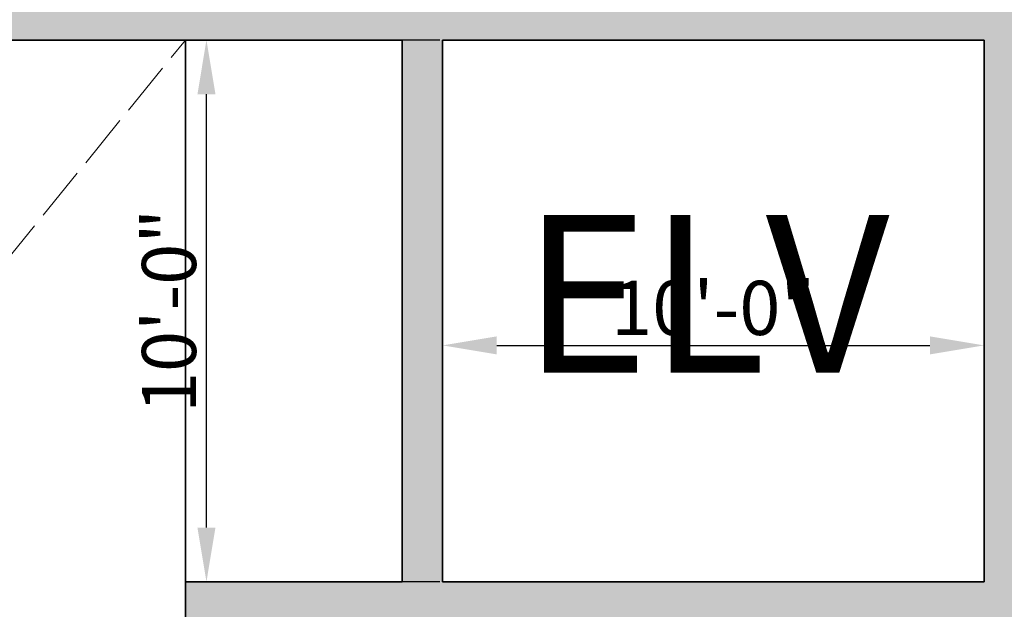
# Model space of a CAD drawing. Units: inches. Extents: x 2083 to 3317, y 1141 to 2115.
# Tile 90 of 256: x 2382 to 2600, y 1577 to 1707. Entities that reach past the tile are written whole.
import ezdxf

# ---------------------------------------------------------------- set-up
doc = ezdxf.new("R2010")
doc.units = ezdxf.units.IN
doc.linetypes.add('ACAD_ISO02W100', pattern=[15, 12, -3])
for name, color, linetype, lineweight in [('A-ANNO-DIMS', 2, 'Continuous', 18), ('A-AREA-IDEN', 7, 'Continuous', 25), ('A-FLOR-OPEN', 8, 'ACAD_ISO02W100', 13), ('A-WALL', 7, 'Continuous', 35)]:
    doc.layers.add(name, color=color, linetype=linetype, lineweight=lineweight)
doc.layers.add('A-WALL-PATT', color=251, linetype='Continuous', lineweight=13, true_color=0x636466)
doc.styles.get("Standard").update_dxf_attribs({"font": 'arial.ttf'})
doc.dimstyles.new('ISO-25', dxfattribs={"dimtxt": 12, "dimasz": 12, "dimexe": 1.25, "dimexo": 0.625, "dimtad": 1, "dimlunit": 3, "dimtxsty": 'Standard', "dimcen": 2.5, "dimadec": 0, "dimazin": 0, "dimtfac": 1, "dimtmove": 0, "dimatfit": 3, "dimfxl": 1, "dimarcsym": 0})

# ---------------------------------------------------------------- blocks, each defined once
blk = doc.blocks.new('*D41')
at = {"layer": 'A-ANNO-DIMS', "color": 0, "lineweight": -2, "transparency": 16777216}
for p, q in [((2475.96, 1583.39), (2475.96, 1636.36)), ((2487.96, 1635.11), (2583.96, 1635.11)), ((2595.96, 1583.39), (2595.96, 1636.36))]:
    blk.add_line(p, q, dxfattribs=at)
at = {"layer": 'A-ANNO-DIMS', "color": 0, "transparency": 16777216}
for points in [[(2487.96, 1637.11), (2487.96, 1633.11), (2475.96, 1635.11)], [(2583.96, 1637.11), (2583.96, 1633.11), (2595.96, 1635.11)]]:
    blk.add_solid(points, dxfattribs=at)
at = {"layer": 'Defpoints', "color": 0, "transparency": 16777216}
for p in [(2595.96, 1635.11), (2475.96, 1582.76), (2595.96, 1582.76)]:
    blk.add_point(p, dxfattribs=at)
at = {"layer": 'A-ANNO-DIMS', "color": 0, "transparency": 16777216, "insert": (2535.96, 1641.86), "char_height": 12, "attachment_point": 5}
blk.add_mtext('10\'-0"', dxfattribs=at)
blk = doc.blocks.new('*D42')
at = {"layer": 'A-ANNO-DIMS', "color": 0, "lineweight": -2, "transparency": 16777216}
for p, q in [((2475.33, 1702.76), (2422.36, 1702.76)), ((2423.61, 1594.76), (2423.61, 1690.76)), ((2475.33, 1582.76), (2422.36, 1582.76))]:
    blk.add_line(p, q, dxfattribs=at)
at = {"layer": 'A-ANNO-DIMS', "color": 0, "transparency": 16777216}
for points in [[(2421.61, 1690.76), (2425.61, 1690.76), (2423.61, 1702.76)], [(2421.61, 1594.76), (2425.61, 1594.76), (2423.61, 1582.76)]]:
    blk.add_solid(points, dxfattribs=at)
at = {"layer": 'Defpoints', "color": 0, "transparency": 16777216}
for p in [(2423.61, 1702.76), (2475.96, 1702.76), (2475.96, 1582.76)]:
    blk.add_point(p, dxfattribs=at)
at = {"layer": 'A-ANNO-DIMS', "color": 0, "transparency": 16777216, "insert": (2416.86, 1642.76), "char_height": 12, "attachment_point": 5, "rotation": 90}
blk.add_mtext('10\'-0"', dxfattribs=at)

msp = doc.modelspace()

# ---------------------------------------------------------------- hatches: boundary and pattern name
at = {"layer": 'A-WALL-PATT'}
h = msp.add_hatch(color=256, dxfattribs=at)
h.dxf.hatch_style = 1
h.paths.add_polyline_path([(3126.96, 2020.761), (2748.96, 2020.761), (2604.96, 2020.761), (2226.96, 2020.761), (2226.96, 1702.761), (2466.96, 1702.761), (2466.96, 1582.761), (2418.96, 1582.761), (2418.96, 1477.761), (2226.96, 1477.761), (2226.96, 1263.261), (2544.96, 1263.261), (2544.96, 1411.761), (2604.96, 1411.761), (2685.96, 1411.761), (2685.96, 1420.761), (2604.96, 1420.761), (2604.96, 1573.761), (2604.96, 1702.761), (2604.96, 2011.761), (2748.96, 2011.761), (2748.96, 1702.761), (2862.96, 1702.761), (2862.96, 1621.761), (2871.96, 1621.761), (2871.96, 1702.761), (2883.96, 1702.761), (2883.96, 1706.939, -0.0264593), (2883.96, 1711.761), (2757.96, 1711.761), (2757.96, 1807.761), (2787.96, 1807.761), (2787.96, 1812.261), (2757.96, 1812.261), (2757.96, 2011.761), (2877.96, 2011.761), (2877.96, 1812.261), (2847.96, 1812.261), (2847.96, 1807.761), (2889.836, 1807.761), (2889.836, 1812.261), (2882.46, 1812.261), (2882.46, 2011.761), (3117.96, 2011.761), (3117.96, 1812.261), (2937.836, 1812.261), (2937.836, 1807.761), (2995.71, 1807.761), (2995.71, 1796.118), (3000.21, 1796.118), (3000.21, 1807.761), (3117.96, 1807.761), (3117.96, 1711.761), (3000.21, 1711.761), (3000.21, 1760.118), (2998.573, 1760.118, -0.020711), (2995.71, 1760.118), (2995.71, 1711.761), (2931.96, 1711.761), (2931.96, 1702.761), (3126.96, 1702.761)])
h.paths.add_polyline_path([(2471.46, 2011.761), (2471.46, 1810.011), (2462.717, 1810.011), (2462.717, 1805.511), (2505.96, 1805.511), (2505.96, 1810.011), (2475.96, 1810.011), (2475.96, 2011.761), (2595.96, 2011.761), (2595.96, 1810.011), (2565.96, 1810.011), (2565.96, 1805.511), (2595.96, 1805.511), (2595.96, 1711.761), (2235.96, 1711.761), (2235.96, 1805.511), (2353.71, 1805.511), (2353.71, 1796.054), (2358.21, 1796.054), (2358.21, 1805.511), (2414.717, 1805.511), (2414.717, 1810.011), (2235.96, 1810.011), (2235.96, 2011.761)], flags=16)
h.paths.add_polyline_path([(2270.205, 1994.61), (2270.205, 1970.61), (2246.205, 1970.61), (2246.205, 1994.61)], flags=0)
edge = h.paths.add_edge_path(flags=0)
edge.add_ellipse((2332.027, 1899.798), major_axis=(-3.043, 3.043), ratio=0.1682525, start_angle=-161.33217, end_angle=-156.30711, ccw=False)
edge.add_ellipse((2333.082, 1898.744), major_axis=(-1.055, 1.055), ratio=0.4535321, start_angle=-123.37102, end_angle=-94.15911)
edge = h.paths.add_edge_path(flags=0)
edge.add_ellipse((2332.027, 1968.876), major_axis=(3.043, 3.043), ratio=0.1682525, start_angle=18.66783, end_angle=23.69289)
edge.add_spline(control_points=[(2332.926, 1970.691), (2332.227, 1970.336), (2330.894, 1969.659), (2328.413, 1970.932), (2327.204, 1967.749), (2324.71, 1969.956), (2322.533, 1967.012), (2320.013, 1971.296), (2317.68, 1968.158), (2316.041, 1967.102), (2315.427, 1966.81)], knot_values=[0, 0, 0, 0, 2.2670587, 4.3245589, 6.6855835, 8.8786411, 11.121502, 14.300359, 17.7552837, 19.732645, 19.732645, 19.732645, 19.732645], degree=3, periodic=0)
edge.add_ellipse((2332.027, 1968.876), major_axis=(3.043, 3.043), ratio=0.1682525, start_angle=18.66783, end_angle=23.69289, ccw=False)
edge.add_ellipse((2333.082, 1969.931), major_axis=(1.055, 1.055), ratio=0.4535321, start_angle=56.62898, end_angle=85.84089, ccw=False)
edge = h.paths.add_edge_path(flags=0)
edge.add_spline(control_points=[(2296.428, 1967.988), (2293.628, 1965.336), (2287.704, 1959.727), (2299.744, 1949.996), (2294.533, 1935.669), (2290.573, 1920.604), (2293.394, 1909.974), (2296.185, 1904.967)], knot_values=[0.0991853, 0.0991853, 0.0991853, 0.0991853, 0.3453009, 0.6198217, 0.9826526, 1.3860932, 1.8105546, 1.8105546, 1.8105546, 1.8105546], degree=3, periodic=0)
edge.add_spline(control_points=[(2296.185, 1904.967), (2297.384, 1902.619), (2298.001, 1901.949), (2298.553, 1901.468)], knot_values=[0.0062457, 0.0062457, 0.0062457, 0.0062457, 0.0554759, 0.0554759, 0.0554759, 0.0554759], degree=3, periodic=0)
edge.add_spline(control_points=[(2298.553, 1901.468), (2297.259, 1900.923), (2295.225, 1900.232), (2293.06, 1900.614), (2292.101, 1900.788), (2292.09, 1900.791)], knot_values=[0.3128349, 0.3128349, 0.3128349, 0.3128349, 0.4017797, 0.4749867, 0.4759027, 0.4759027, 0.4759027, 0.4759027], degree=3, periodic=0)
edge.add_arc((2292.794, 1904.664), 3.937, 215.4209, 259.69818, ccw=False)
edge.add_spline(control_points=[(2289.585, 1902.382), (2289.477, 1902.535), (2289.368, 1902.688), (2289.261, 1902.841)], knot_values=[0.1028719, 0.1028719, 0.1028719, 0.1028719, 0.1168958, 0.1168958, 0.1168958, 0.1168958], degree=3, periodic=0)
edge.add_spline(control_points=[(2289.261, 1902.841), (2288.687, 1902.55), (2287.64, 1902.02), (2285.881, 1901.874), (2283.853, 1901.504), (2281.72, 1899.711), (2278.467, 1899.493), (2276.157, 1901.883), (2272.259, 1899.804), (2267.778, 1901.843), (2262.244, 1900.184), (2257.415, 1901.782), (2254.318, 1900.726), (2253.178, 1900.337)], knot_values=[0, 0, 0, 0, 1.9079767, 3.4771759, 5.261074, 7.9728515, 11.6802485, 13.7179214, 16.9395917, 22.789562, 27.5025027, 33.5952153, 37.1456181, 37.1456181, 37.1456181, 37.1456181], degree=3, periodic=0)
edge.add_line((2253.178, 1900.337), (2250.244, 1902.841))
edge.add_line((2250.244, 1902.841), (2250.244, 1965.833))
edge.add_line((2250.244, 1965.833), (2253.178, 1968.337))
edge.add_spline(control_points=[(2253.178, 1968.337), (2254.318, 1967.948), (2257.415, 1966.892), (2262.244, 1968.49), (2267.778, 1966.831), (2271.527, 1968.537), (2273.876, 1967.828), (2274.207, 1967.728)], knot_values=[0, 0, 0, 0, 0.0901802, 0.2449351, 0.3646438, 0.5132331, 0.5378548, 0.5378548, 0.5378548, 0.5378548], degree=3, periodic=0)
edge.add_arc((2274.353, 1963.793), 3.937, 72.05113, 92.12795, ccw=False)
edge.add_arc((2281.297, 1985.23), 18.596, 252.05113, 288.56572)
edge.add_arc((2292.317, 1956.029), 12.646, 71.02679, 113.77822, ccw=False)
edge = h.paths.add_edge_path(flags=0)
edge.add_spline(control_points=[(2274.899, 1951.856), (2275.066, 1951.617), (2275.233, 1951.377), (2275.398, 1951.136)], knot_values=[1.4099157, 1.4099157, 1.4099157, 1.4099157, 1.4315903, 1.4315903, 1.4315903, 1.4315903], degree=3, periodic=0)
edge.add_spline(control_points=[(2275.398, 1951.136), (2275.792, 1950.562), (2276.179, 1949.984), (2276.546, 1949.397)], knot_values=[1.3582378, 1.3582378, 1.3582378, 1.3582378, 1.4099157, 1.4099157, 1.4099157, 1.4099157], degree=3, periodic=0)
edge.add_line((2276.546, 1949.397), (2277.437, 1947.862))
edge.add_spline(control_points=[(2277.437, 1947.862), (2276.304, 1945.673), (2274.64, 1942.427), (2274.632, 1938.094), (2272.799, 1930.852), (2274.356, 1943.897), (2275.948, 1947.923), (2276.546, 1949.397)], knot_values=[0.0056315, 0.0056315, 0.0056315, 0.0056315, 0.1860139, 0.2660015, 0.3570872, 0.5963902, 0.7397317, 0.7397317, 0.7397317, 0.7397317], degree=3, periodic=0)
edge.add_spline(control_points=[(2276.546, 1949.397), (2276.179, 1949.984), (2275.792, 1950.562), (2275.398, 1951.136)], knot_values=[1.3582378, 1.3582378, 1.3582378, 1.3582378, 1.4099157, 1.4099157, 1.4099157, 1.4099157], degree=3, periodic=0)
edge.add_spline(control_points=[(2275.398, 1951.136), (2274.943, 1950.08), (2274.208, 1948.025), (2273.935, 1944.851), (2272.469, 1937.627), (2273.466, 1945.696), (2274.701, 1951.059), (2274.899, 1951.856)], knot_values=[0.1043639, 0.1043639, 0.1043639, 0.1043639, 0.1896363, 0.2696239, 0.3607096, 0.6000126, 0.6446217, 0.6446217, 0.6446217, 0.6446217], degree=3, periodic=0)
h.paths.add_polyline_path([(2269.168, 1963.128, -0.3575267), (2268.171, 1960.976, -0.0925607), (2268.171, 1939.436, -0.3575267), (2269.168, 1937.285, -0.3575267), (2267.016, 1938.282, -0.1647847), (2254.686, 1938.282, -0.3575267), (2252.534, 1937.285, -0.3575267), (2253.531, 1939.436, -0.0925607), (2253.531, 1960.976, -0.3575267), (2252.534, 1963.128, -0.3575267), (2254.686, 1962.131, -0.1647847), (2267.016, 1962.131, -0.3575267)], flags=0)
h.paths.add_polyline_path([(2248.874, 1967.802), (2248.874, 1957.028), (2249.458, 1957.028), (2249.458, 1911.647), (2248.874, 1911.647), (2248.874, 1900.873), (2246.512, 1900.873, 0.1973271), (2244.15, 1902.457), (2244.15, 1966.218, 0.1973271), (2246.512, 1967.802)], flags=0)
h.paths.add_polyline_path([(2269.168, 1931.389, -0.3575267), (2268.171, 1929.238, -0.0925607), (2268.171, 1907.698, -0.3575267), (2269.168, 1905.547, -0.3575267), (2267.016, 1906.544, -0.1647847), (2254.686, 1906.544, -0.3575267), (2252.534, 1905.547, -0.3575267), (2253.531, 1907.698, -0.0925607), (2253.531, 1929.238, -0.3575267), (2252.534, 1931.389, -0.3575267), (2254.686, 1930.392, -0.1647847), (2267.016, 1930.392, -0.3575267)], flags=0)
edge = h.paths.add_edge_path(flags=0)
edge.add_spline(control_points=[(2276.197, 1906.724), (2276.168, 1909.029), (2276.114, 1913.372), (2270.598, 1924.925), (2273.905, 1919.013), (2275.922, 1916.262), (2275.475, 1912.402), (2277.258, 1910.381), (2276.696, 1908.225), (2276.646, 1906.813), (2276.618, 1906.008)], knot_values=[0, 0, 0, 0, 8.6102597, 16.2212739, 18.8430575, 23.8048978, 27.4408283, 29.3561016, 31.2034776, 33.6506866, 33.6506866, 33.6506866, 33.6506866], degree=3, periodic=0)
edge.add_spline(control_points=[(2276.618, 1906.008), (2276.623, 1905.624), (2276.498, 1904.629), (2275.442, 1903.855), (2274.937, 1903.08), (2274.859, 1902.841)], knot_values=[0.1564884, 0.1564884, 0.1564884, 0.1564884, 0.1843975, 0.2313765, 0.2505985, 0.2505985, 0.2505985, 0.2505985], degree=3, periodic=0)
edge.add_line((2274.859, 1902.841), (2276.506, 1902.841))
edge.add_spline(control_points=[(2276.506, 1902.841), (2276.788, 1903.085), (2277.665, 1904.125), (2278.25, 1904.341), (2277.654, 1908.527), (2278.156, 1906.228), (2278.1, 1905.286), (2278.847, 1904.069), (2277.857, 1903.415), (2277.874, 1902.991), (2277.904, 1902.841)], knot_values=[0.0595743, 0.0595743, 0.0595743, 0.0595743, 0.0807529, 0.1037415, 0.1697201, 0.1760361, 0.2071372, 0.2404744, 0.2623409, 0.2736605, 0.2736605, 0.2736605, 0.2736605], degree=3, periodic=0)
edge.add_line((2277.904, 1902.841), (2280.03, 1902.841))
edge.add_spline(control_points=[(2280.03, 1902.841), (2279.888, 1903.088), (2279.499, 1903.982), (2280.152, 1905.939), (2278.104, 1909.658), (2279.762, 1907.185), (2280.328, 1904.875), (2280.485, 1903.49), (2281.463, 1903.249), (2281.758, 1902.936), (2281.834, 1902.841)], knot_values=[0.013856, 0.013856, 0.013856, 0.013856, 0.0348738, 0.0888667, 0.1078792, 0.1267378, 0.158714, 0.1937575, 0.2174868, 0.2267221, 0.2267221, 0.2267221, 0.2267221], degree=3, periodic=0)
edge.add_spline(control_points=[(2281.834, 1902.841), (2281.788, 1902.827), (2281.647, 1902.783), (2281.396, 1902.859), (2281.088, 1902.985), (2280.721, 1903.061), (2280.333, 1903.026), (2280.125, 1902.899), (2280.03, 1902.841)], knot_values=[0, 0, 0, 0, 0.1441304, 0.435517, 0.7492759, 1.1530457, 1.5483707, 1.878348, 1.878348, 1.878348, 1.878348], degree=3, periodic=0)
edge.add_line((2280.03, 1902.841), (2277.904, 1902.841))
edge.add_spline(control_points=[(2277.904, 1902.841), (2277.893, 1902.796), (2277.865, 1902.68), (2277.607, 1902.687), (2277.274, 1902.801), (2276.838, 1902.62), (2276.584, 1902.789), (2276.506, 1902.841)], knot_values=[0, 0, 0, 0, 0.1271885, 0.3261988, 0.6280094, 1.2435704, 1.5153306, 1.5153306, 1.5153306, 1.5153306], degree=3, periodic=0)
edge.add_line((2276.506, 1902.841), (2274.859, 1902.841))
edge.add_spline(control_points=[(2274.859, 1902.841), (2274.814, 1902.899), (2274.725, 1903.013), (2274.493, 1903.119), (2274.244, 1902.961), (2273.937, 1903.185), (2273.614, 1902.983), (2273.408, 1902.883), (2273.322, 1902.841)], knot_values=[0, 0, 0, 0, 0.2184302, 0.4369566, 0.6879766, 0.9903786, 1.3983955, 1.6918498, 1.6918498, 1.6918498, 1.6918498], degree=3, periodic=0)
edge.add_spline(control_points=[(2273.322, 1902.841), (2273.617, 1903.446), (2274.274, 1904.538), (2276.027, 1904.574), (2276.207, 1906.584), (2276.197, 1906.724)], knot_values=[0.0122268, 0.0122268, 0.0122268, 0.0122268, 0.0594721, 0.1062177, 0.134458, 0.134458, 0.134458, 0.134458], degree=3, periodic=0)
h.paths.add_polyline_path([(2270.776, 1897.79), (2270.776, 1873.79), (2246.776, 1873.79), (2246.776, 1897.79)], flags=0)
h.paths.add_polyline_path([(2353.71, 1760.005), (2353.71, 1760.054), (2358.21, 1760.054, -0.033729)], flags=0)
h.paths.add_polyline_path([(2321.819, 1737.529), (2341.995, 1737.529, -0.4142136), (2343.203, 1736.321), (2343.203, 1721.021, -0.4142136), (2341.995, 1719.813), (2321.819, 1719.813, -0.4142136), (2320.611, 1721.021), (2320.611, 1736.321, -0.4142136)], flags=0)
h.paths.add_polyline_path([(2324.235, 1736.321), (2339.579, 1736.321, -0.4142136), (2341.995, 1733.905), (2341.995, 1725.45, -0.4142136), (2339.579, 1723.034), (2333.681, 1723.034), (2333.845, 1722.045, -0.8706461), (2335.425, 1721.826, -0.767327), (2333.923, 1721.423), (2331.291, 1721.423, -0.767327), (2329.788, 1721.826, -0.8706461), (2331.368, 1722.045), (2331.533, 1723.034), (2324.235, 1723.034, -0.4142136), (2321.819, 1725.45), (2321.819, 1733.905, -0.4142136)], flags=0)
h.paths.add_polyline_path([(2570.484, 1928.615), (2589.684, 1928.615), (2590.169, 1928.615), (2590.169, 1904.993), (2570.484, 1904.993)], flags=0)
h.paths.add_polyline_path([(2574.447, 1927.264, -1), (2572.829, 1927.264, -1)], flags=0)
h.paths.add_polyline_path([(2573.09, 1926.941), (2573.925, 1927.776), (2574.148, 1927.553), (2573.313, 1926.718)], flags=0)
h.paths.add_polyline_path([(2578.779, 1919.73, -1), (2571.592, 1919.73, -1)], flags=0)
h.paths.add_polyline_path([(2578.385, 1919.73, -1), (2571.985, 1919.73, -1)], flags=0)
h.paths.add_polyline_path([(2331.596, 1729.476, -1), (2333.618, 1729.476, -1)], flags=0)
h.paths.add_polyline_path([(2578.034, 1927.264, -1), (2576.416, 1927.264, -1)], flags=0)
h.paths.add_polyline_path([(2576.689, 1927.531), (2576.912, 1927.754), (2577.747, 1926.919), (2577.524, 1926.696)], flags=0)
h.paths.add_polyline_path([(2578.139, 1909.86, -1), (2572.232, 1909.86, -1)], flags=0)
h.paths.add_polyline_path([(2577.745, 1909.86, -1), (2572.625, 1909.86, -1)], flags=0)
h.paths.add_polyline_path([(2583.798, 1927.264, -1), (2582.179, 1927.264, -1)], flags=0)
h.paths.add_polyline_path([(2582.719, 1927.754), (2583.554, 1926.919), (2583.331, 1926.696), (2582.496, 1927.531)], flags=0)
h.paths.add_polyline_path([(2582.496, 1927.531), (2582.719, 1927.754), (2583.554, 1926.919), (2583.331, 1926.696)], flags=0)
h.paths.add_polyline_path([(2587.739, 1920.53, -1), (2581.832, 1920.53, -1)], flags=0)
h.paths.add_polyline_path([(2587.345, 1920.53, -1), (2582.225, 1920.53, -1)], flags=0)
h.paths.add_polyline_path([(2587.385, 1927.264, -1), (2585.766, 1927.264, -1)], flags=0)
h.paths.add_polyline_path([(2586.082, 1926.98), (2586.917, 1927.815), (2587.14, 1927.593), (2586.305, 1926.758)], flags=0)
h.paths.add_polyline_path([(2588.379, 1910.66, -1), (2581.192, 1910.66, -1)], flags=0)
h.paths.add_polyline_path([(2587.985, 1910.66, -1), (2581.585, 1910.66, -1)], flags=0)
h.paths.add_polyline_path([(2417.168, 1729.478), (2437.344, 1729.478, -0.4142136), (2438.552, 1728.27), (2438.552, 1712.969, -0.4142136), (2437.344, 1711.761), (2417.168, 1711.761, -0.4142136), (2415.96, 1712.969), (2415.96, 1728.27, -0.4142136)], flags=0)
h.paths.add_polyline_path([(2419.584, 1728.27), (2434.928, 1728.27, -0.4142136), (2437.344, 1725.854), (2437.344, 1717.398, -0.4142136), (2434.928, 1714.983), (2429.029, 1714.983), (2429.194, 1713.994, -0.8706461), (2430.774, 1713.775, -0.767327), (2429.271, 1713.372), (2426.64, 1713.372, -0.767327), (2425.137, 1713.775, -0.8706461), (2426.717, 1713.994), (2426.882, 1714.983), (2419.584, 1714.983, -0.4142136), (2417.168, 1717.398), (2417.168, 1725.854, -0.4142136)], flags=0)
h.paths.add_polyline_path([(2419.584, 1728.27), (2434.928, 1728.27, -0.4142136), (2437.344, 1725.854), (2437.344, 1717.398, -0.4142136), (2434.928, 1714.983), (2429.029, 1714.983), (2428.358, 1719.009), (2427.553, 1719.009), (2426.882, 1714.983), (2419.584, 1714.983, -0.4142136), (2417.168, 1717.398), (2417.168, 1725.854, -0.4142136)], flags=0)
h.paths.add_polyline_path([(2426.944, 1721.425, -1), (2428.967, 1721.425, -1)], flags=0)
h.paths.add_polyline_path([(2475.96, 1702.761), (2595.96, 1702.761), (2595.96, 1582.761), (2475.96, 1582.761)], flags=16)
h.paths.add_polyline_path([(2427.96, 1573.761), (2595.96, 1573.761), (2595.96, 1468.761), (2595.96, 1420.761), (2384.46, 1420.761), (2384.46, 1468.761), (2427.96, 1468.761)], flags=16)
h.paths.add_polyline_path([(2379.96, 1468.761), (2379.96, 1420.761), (2235.96, 1420.761), (2235.96, 1468.761)], flags=16)
h.paths.add_polyline_path([(2317.816, 1466.696), (2337.992, 1466.696, -0.4142136), (2339.2, 1465.488), (2339.2, 1450.187, -0.4142136), (2337.992, 1448.979), (2317.816, 1448.979, -0.4142136), (2316.608, 1450.187), (2316.608, 1465.488, -0.4142136)], flags=0)
h.paths.add_polyline_path([(2320.232, 1465.488), (2335.576, 1465.488, -0.4142136), (2337.992, 1463.072), (2337.992, 1454.616, -0.4142136), (2335.576, 1452.2), (2329.677, 1452.2), (2329.842, 1451.212, -0.8706461), (2331.422, 1450.992, -0.767327), (2329.92, 1450.59), (2327.288, 1450.59, -0.767327), (2325.785, 1450.992, -0.8706461), (2327.365, 1451.212), (2327.53, 1452.2), (2320.232, 1452.2, -0.4142136), (2317.816, 1454.616), (2317.816, 1463.072, -0.4142136)], flags=0)
h.paths.add_polyline_path([(2320.232, 1465.488), (2335.576, 1465.488, -0.4142136), (2337.992, 1463.072), (2337.992, 1454.616, -0.4142136), (2335.576, 1452.2), (2329.677, 1452.2), (2329.006, 1456.227), (2328.201, 1456.227), (2327.53, 1452.2), (2320.232, 1452.2, -0.4142136), (2317.816, 1454.616), (2317.816, 1463.072, -0.4142136)], flags=0)
h.paths.add_polyline_path([(2327.593, 1458.643, -1), (2329.615, 1458.643, -1)], flags=0)
h.paths.add_polyline_path([(2244.412, 1433.34), (2241.921, 1433.34, -0.4142136), (2240.018, 1435.244), (2240.018, 1440.953, -0.4142105), (2241.921, 1442.856), (2244.412, 1442.856, -1.9764724)], flags=0)
h.paths.add_polyline_path([(2245.357, 1434.398, -0.4142136), (2245.357, 1441.799, -2.1440985)], flags=0)
h.paths.add_polyline_path([(2535.96, 1416.261), (2535.96, 1272.261), (2235.96, 1272.261), (2235.96, 1416.261)], flags=16)
h.paths.add_polyline_path([(2260.12, 1384.293), (2260.12, 1362.039), (2237.865, 1362.039), (2237.865, 1384.293)], flags=0)
edge = h.paths.add_edge_path(flags=0)
edge.add_line((2318.252, 1362.093), (2318.146, 1362.001))
edge.add_ellipse((2317.445, 1360.431), major_axis=(2.822, 2.822), ratio=0.1682525, start_angle=18.66783, end_angle=20.94813, ccw=False)
edge.add_ellipse((2318.423, 1361.409), major_axis=(0.978, 0.978), ratio=0.4535321, start_angle=56.62898, end_angle=70.2262, ccw=False)
edge = h.paths.add_edge_path(flags=0)
edge.add_line((2319.107, 1295.571), (2319.015, 1295.677))
edge.add_ellipse((2317.445, 1296.378), major_axis=(-2.822, 2.822), ratio=0.1682525, start_angle=-161.33217, end_angle=-159.05187, ccw=False)
edge.add_ellipse((2318.423, 1295.4), major_axis=(-0.978, 0.978), ratio=0.4535321, start_angle=-123.37102, end_angle=-109.7738)
edge = h.paths.add_edge_path(flags=0)
edge.add_spline(control_points=[(2284.21, 1301.17), (2284.581, 1300.445), (2284.891, 1299.892), (2285.16, 1299.461)], knot_values=[0.0390658, 0.0390658, 0.0390658, 0.0390658, 0.0554759, 0.0554759, 0.0554759, 0.0554759], degree=3, periodic=0)
edge.add_line((2285.16, 1299.461), (2284.21, 1301.17))
edge = h.paths.add_edge_path(flags=0)
edge.add_line((2280.412, 1297.298), (2283.37, 1297.036))
edge.add_line((2283.37, 1297.036), (2286.406, 1297.926))
edge.add_spline(control_points=[(2286.406, 1297.926), (2285.305, 1297.463), (2284.345, 1297.129), (2283.37, 1297.036)], knot_values=[0.3943688, 0.3943688, 0.3943688, 0.3943688, 0.4759027, 0.4759027, 0.4759027, 0.4759027], degree=3, periodic=0)
edge.add_spline(control_points=[(2283.37, 1297.036), (2283.281, 1297.028), (2282.316, 1296.957), (2281.313, 1297.134), (2280.423, 1297.296), (2280.412, 1297.298)], knot_values=[0.3128349, 0.3128349, 0.3128349, 0.3128349, 0.3202458, 0.3934528, 0.3943688, 0.3943688, 0.3943688, 0.3943688], degree=3, periodic=0)
edge = h.paths.add_edge_path(flags=0)
edge.add_line((2284.436, 1359.607), (2280.446, 1355.328))
edge.add_line((2280.446, 1355.328), (2279.58, 1351.018))
edge.add_line((2279.58, 1351.018), (2282.413, 1346.58))
edge.add_spline(control_points=[(2282.413, 1346.58), (2283.153, 1345.589), (2284.253, 1344.029), (2284.801, 1342.387), (2284.935, 1341.806)], knot_values=[1.2400982, 1.2400982, 1.2400982, 1.2400982, 1.3328922, 1.3827123, 1.3827123, 1.3827123, 1.3827123], degree=3, periodic=0)
edge.add_spline(control_points=[(2284.935, 1341.806), (2285.319, 1340.141), (2285.233, 1338.409), (2284.91, 1336.654)], knot_values=[1.0974841, 1.0974841, 1.0974841, 1.0974841, 1.2400982, 1.2400982, 1.2400982, 1.2400982], degree=3, periodic=0)
edge.add_spline(control_points=[(2284.91, 1336.654), (2284.587, 1334.899), (2284.027, 1333.12), (2283.463, 1331.361)], knot_values=[0.9548699, 0.9548699, 0.9548699, 0.9548699, 1.0974841, 1.0974841, 1.0974841, 1.0974841], degree=3, periodic=0)
edge.add_line((2283.463, 1331.361), (2281.89, 1326.153))
edge.add_line((2281.89, 1326.153), (2280.756, 1321.056))
edge.add_line((2280.756, 1321.056), (2280.299, 1316.002))
edge.add_line((2280.299, 1316.002), (2280.716, 1310.95))
edge.add_line((2280.716, 1310.95), (2282.028, 1305.972))
edge.add_line((2282.028, 1305.972), (2284.21, 1301.17))
edge.add_spline(control_points=[(2284.21, 1301.17), (2283.341, 1302.73), (2282.612, 1304.336), (2282.028, 1305.972)], knot_values=[0.0991853, 0.0991853, 0.0991853, 0.0991853, 0.2417994, 0.2417994, 0.2417994, 0.2417994], degree=3, periodic=0)
edge.add_spline(control_points=[(2282.028, 1305.972), (2281.444, 1307.608), (2281.005, 1309.273), (2280.716, 1310.95)], knot_values=[0.2417994, 0.2417994, 0.2417994, 0.2417994, 0.3844135, 0.3844135, 0.3844135, 0.3844135], degree=3, periodic=0)
edge.add_spline(control_points=[(2280.716, 1310.95), (2280.433, 1312.588), (2280.289, 1314.277), (2280.299, 1315.962), (2280.299, 1316.002)], knot_values=[0.3844135, 0.3844135, 0.3844135, 0.3844135, 0.5236467, 0.5270276, 0.5270276, 0.5270276, 0.5270276], degree=3, periodic=0)
edge.add_spline(control_points=[(2280.299, 1316.002), (2280.312, 1317.687), (2280.478, 1319.368), (2280.756, 1321.056)], knot_values=[0.5270276, 0.5270276, 0.5270276, 0.5270276, 0.6696417, 0.6696417, 0.6696417, 0.6696417], degree=3, periodic=0)
edge.add_spline(control_points=[(2280.756, 1321.056), (2281.035, 1322.744), (2281.426, 1324.44), (2281.89, 1326.153)], knot_values=[0.6696417, 0.6696417, 0.6696417, 0.6696417, 0.8122558, 0.8122558, 0.8122558, 0.8122558], degree=3, periodic=0)
edge.add_spline(control_points=[(2281.89, 1326.153), (2282.264, 1327.533), (2282.788, 1329.262), (2283.353, 1331.018), (2283.463, 1331.361)], knot_values=[0.8122558, 0.8122558, 0.8122558, 0.8122558, 0.9270873, 0.9548699, 0.9548699, 0.9548699, 0.9548699], degree=3, periodic=0)
edge.add_line((2283.463, 1331.361), (2284.91, 1336.654))
edge.add_line((2284.91, 1336.654), (2284.935, 1341.806))
edge.add_line((2284.935, 1341.806), (2282.413, 1346.58))
edge.add_spline(control_points=[(2282.413, 1346.58), (2281.275, 1348.104), (2280.078, 1349.57), (2279.58, 1351.018)], knot_values=[1.3827123, 1.3827123, 1.3827123, 1.3827123, 1.5253264, 1.5253264, 1.5253264, 1.5253264], degree=3, periodic=0)
edge.add_spline(control_points=[(2279.58, 1351.018), (2279.443, 1351.415), (2279.136, 1352.857), (2279.735, 1354.29), (2280.446, 1355.328)], knot_values=[1.5253264, 1.5253264, 1.5253264, 1.5253264, 1.564439, 1.6679405, 1.6679405, 1.6679405, 1.6679405], degree=3, periodic=0)
edge.add_spline(control_points=[(2280.446, 1355.328), (2281.426, 1356.758), (2282.931, 1358.183), (2284.436, 1359.607)], knot_values=[1.6679405, 1.6679405, 1.6679405, 1.6679405, 1.8105546, 1.8105546, 1.8105546, 1.8105546], degree=3, periodic=0)
edge.add_arc((2280.623, 1348.518), 11.726, 71.02679, 113.77822)
edge.add_arc((2270.405, 1375.595), 17.244, 252.05113, 288.56572, ccw=False)
edge.add_arc((2263.966, 1355.718), 3.651, 72.05113, 92.12795)
edge.add_arc((2263.966, 1355.718), 3.651, 92.12795, 177.98513)
edge.add_spline(control_points=[(2260.318, 1355.846), (2260.26, 1354.221), (2260.551, 1350.187), (2262.999, 1346.766), (2264.473, 1344.649)], knot_values=[1.4315903, 1.4315903, 1.4315903, 1.4315903, 1.5641438, 1.7706953, 1.7706953, 1.7706953, 1.7706953], degree=3, periodic=0)
edge.add_line((2264.473, 1344.649), (2264.936, 1343.983))
edge.add_spline(control_points=[(2263.801, 1340.248), (2263.843, 1340.514), (2264.067, 1341.756), (2264.513, 1343.002), (2264.935, 1343.981)], knot_values=[0.5365702, 0.5365702, 0.5365702, 0.5365702, 0.5593494, 0.6446217, 0.6446217, 0.6446217, 0.6446217], degree=3, periodic=0)
edge.add_spline(control_points=[(2264.935, 1343.981), (2265.118, 1343.715), (2265.299, 1343.448), (2265.477, 1343.179)], knot_values=[1.3840767, 1.3840767, 1.3840767, 1.3840767, 1.4099157, 1.4099157, 1.4099157, 1.4099157], degree=3, periodic=0)
edge.add_spline(control_points=[(2265.477, 1343.179), (2265.655, 1342.911), (2265.829, 1342.641), (2265.999, 1342.369)], knot_values=[1.3582378, 1.3582378, 1.3582378, 1.3582378, 1.3840767, 1.3840767, 1.3840767, 1.3840767], degree=3, periodic=0)
edge.add_line((2265.999, 1342.369), (2266.826, 1340.946))
edge.add_spline(control_points=[(2266.826, 1340.946), (2268.894, 1337.09), (2271.398, 1325.843), (2270.516, 1310.569), (2275.919, 1301.861), (2277.79, 1299.199)], knot_values=[0.1168958, 0.1168958, 0.1168958, 0.1168958, 0.4729873, 1.0509689, 1.3137934, 1.3137934, 1.3137934, 1.3137934], degree=3, periodic=0)
edge.add_spline(control_points=[(2277.79, 1299.199), (2277.839, 1299.128), (2277.889, 1299.057), (2277.94, 1298.987)], knot_values=[0.1098839, 0.1098839, 0.1098839, 0.1098839, 0.1168958, 0.1168958, 0.1168958, 0.1168958], degree=3, periodic=0)
edge.add_line((2277.94, 1298.987), (2277.789, 1299.199))
edge.add_spline(control_points=[(2277.789, 1299.199), (2277.257, 1298.929), (2276.286, 1298.438), (2275.039, 1298.334), (2274.383, 1298.239), (2274.215, 1298.209)], knot_values=[33.1218702, 33.1218702, 33.1218702, 33.1218702, 35.0290557, 36.5982549, 37.1448269, 37.1448269, 37.1448269, 37.1448269], degree=3, periodic=0)
edge.add_line((2274.215, 1298.209), (2273.073, 1297.893))
edge.add_spline(control_points=[(2273.073, 1297.893), (2272.323, 1297.58), (2271.039, 1296.511), (2269.248, 1296.226), (2268.423, 1296.375)], knot_values=[26.5325843, 26.5325843, 26.5325843, 26.5325843, 29.198919, 31.8391012, 31.8391012, 31.8391012, 31.8391012], degree=3, periodic=0)
edge.add_line((2268.423, 1296.375), (2263.879, 1297.458))
edge.add_spline(control_points=[(2263.879, 1297.458), (2263.556, 1297.359), (2261.86, 1296.839), (2260.239, 1297.282), (2258.933, 1297.516)], knot_values=[15.9195506, 15.9195506, 15.9195506, 15.9195506, 16.9395917, 21.2260675, 21.2260675, 21.2260675, 21.2260675], degree=3, periodic=0)
edge.add_line((2258.933, 1297.516), (2254.055, 1297.329))
edge.add_spline(control_points=[(2254.055, 1297.329), (2253.756, 1297.296), (2252.114, 1297.165), (2250.462, 1297.544), (2249.13, 1297.668)], knot_values=[5.3065169, 5.3065169, 5.3065169, 5.3065169, 6.2764352, 10.6130337, 10.6130337, 10.6130337, 10.6130337], degree=3, periodic=0)
edge.add_line((2249.13, 1297.668), (2244.332, 1296.878))
edge.add_line((2244.332, 1296.878), (2241.611, 1299.199))
edge.add_line((2241.611, 1299.199), (2241.611, 1357.609))
edge.add_line((2241.611, 1357.609), (2244.332, 1359.931))
edge.add_line((2244.332, 1359.931), (2252.729, 1359.543))
edge.add_spline(control_points=[(2252.729, 1359.543), (2252.871, 1359.546), (2253.306, 1359.548), (2253.74, 1359.514), (2254.032, 1359.482)], knot_values=[0.233291, 0.233291, 0.233291, 0.233291, 0.2449351, 0.2689274, 0.2689274, 0.2689274, 0.2689274], degree=3, periodic=0)
edge.add_line((2254.032, 1359.482), (2259.587, 1359.416))
edge.add_spline(control_points=[(2259.587, 1359.416), (2260.677, 1359.629), (2262.073, 1359.897), (2263.524, 1359.459), (2263.83, 1359.366)], knot_values=[0.4225164, 0.4225164, 0.4225164, 0.4225164, 0.5132331, 0.5378548, 0.5378548, 0.5378548, 0.5378548], degree=3, periodic=0)
edge.add_arc((2263.966, 1355.718), 3.651, 72.05113, 92.12795, ccw=False)
edge.add_arc((2270.405, 1375.595), 17.244, 252.05113, 288.56572)
edge.add_arc((2280.623, 1348.518), 11.726, 71.02679, 113.77822, ccw=False)
h.paths.add_polyline_path([(2240.341, 1359.435), (2240.341, 1349.444), (2240.882, 1349.444), (2240.882, 1307.365), (2240.341, 1307.365), (2240.341, 1297.374), (2238.15, 1297.374, 0.1973271), (2235.96, 1298.843), (2235.96, 1357.966, 0.1973271), (2238.15, 1359.435)], flags=0)
h.paths.add_polyline_path([(2259.158, 1355.101, -0.3575267), (2258.233, 1353.106, -0.0925607), (2258.233, 1333.133, -0.3575267), (2259.158, 1331.138, -0.3575267), (2257.163, 1332.062, -0.1647847), (2245.729, 1332.062, -0.3575267), (2243.735, 1331.138, -0.3575267), (2244.659, 1333.133, -0.0925607), (2244.659, 1353.106, -0.3575267), (2243.735, 1355.101, -0.3575267), (2245.729, 1354.176, -0.1647847), (2257.163, 1354.176, -0.3575267)], flags=0)
edge = h.paths.add_edge_path(flags=0)
edge.add_line((2265.999, 1342.369), (2266.826, 1340.946))
edge.add_line((2266.826, 1340.946), (2265.308, 1337.814))
edge.add_line((2265.308, 1337.814), (2264.358, 1334.653))
edge.add_line((2264.358, 1334.653), (2264.262, 1333.8))
edge.add_spline(control_points=[(2264.262, 1333.8), (2264.208, 1333.187), (2264.162, 1332.366), (2264.007, 1331.414), (2263.969, 1331.202)], knot_values=[0.4644442, 0.4644442, 0.4644442, 0.4644442, 0.5166905, 0.5316081, 0.5316081, 0.5316081, 0.5316081], degree=3, periodic=0)
edge.add_spline(control_points=[(2263.969, 1331.202), (2263.775, 1330.119), (2263.424, 1328.791), (2263.257, 1328.531), (2263.234, 1328.515)], knot_values=[0.3726816, 0.3726816, 0.3726816, 0.3726816, 0.4488497, 0.4644442, 0.4644442, 0.4644442, 0.4644442], degree=3, periodic=0)
edge.add_spline(control_points=[(2263.234, 1328.515), (2263.096, 1328.42), (2263.131, 1329.301), (2263.275, 1330.616)], knot_values=[0.2809191, 0.2809191, 0.2809191, 0.2809191, 0.3726816, 0.3726816, 0.3726816, 0.3726816], degree=3, periodic=0)
edge.add_spline(control_points=[(2263.275, 1330.616), (2263.419, 1331.93), (2263.672, 1333.677), (2263.97, 1335.315)], knot_values=[0.1891566, 0.1891566, 0.1891566, 0.1891566, 0.2809191, 0.2809191, 0.2809191, 0.2809191], degree=3, periodic=0)
edge.add_spline(control_points=[(2263.97, 1335.315), (2264.1, 1336.032), (2264.419, 1337.622), (2264.755, 1338.864), (2264.947, 1339.491)], knot_values=[0.097394, 0.097394, 0.097394, 0.097394, 0.1375775, 0.1891566, 0.1891566, 0.1891566, 0.1891566], degree=3, periodic=0)
edge.add_spline(control_points=[(2264.947, 1339.491), (2265.29, 1340.606), (2265.644, 1341.494), (2265.999, 1342.369)], knot_values=[0.0056315, 0.0056315, 0.0056315, 0.0056315, 0.097394, 0.097394, 0.097394, 0.097394], degree=3, periodic=0)
h.paths.add_polyline_path([(2259.158, 1325.671, -0.3575267), (2258.233, 1323.676, -0.0925607), (2258.233, 1303.703, -0.3575267), (2259.158, 1301.708, -0.3575267), (2257.163, 1302.633, -0.1647847), (2245.729, 1302.633, -0.3575267), (2243.735, 1301.708, -0.3575267), (2244.659, 1303.703, -0.0925607), (2244.659, 1323.676, -0.3575267), (2243.735, 1325.671, -0.3575267), (2245.729, 1324.747, -0.1647847), (2257.163, 1324.747, -0.3575267)], flags=0)
edge = h.paths.add_edge_path(flags=0)
edge.add_spline(control_points=[(2261.709, 1317.311), (2261.679, 1317.418), (2261.762, 1317.389), (2262.491, 1316.09), (2262.962, 1315.301)], knot_values=[14.9558607, 14.9558607, 14.9558607, 14.9558607, 16.2212739, 18.6948259, 18.6948259, 18.6948259, 18.6948259], degree=3, periodic=0)
edge.add_spline(control_points=[(2262.962, 1315.301), (2262.99, 1315.254), (2263.702, 1314.067), (2264.349, 1313.127), (2264.73, 1312.164)], knot_values=[18.6948259, 18.6948259, 18.6948259, 18.6948259, 18.8430575, 22.433791, 22.433791, 22.433791, 22.433791], degree=3, periodic=0)
edge.add_spline(control_points=[(2264.73, 1312.164), (2264.876, 1311.796), (2265.177, 1310.77), (2265.143, 1309.559), (2265.248, 1308.824)], knot_values=[22.433791, 22.433791, 22.433791, 22.433791, 23.8048978, 26.1727562, 26.1727562, 26.1727562, 26.1727562], degree=3, periodic=0)
edge.add_line((2265.248, 1308.824), (2265.851, 1307.172))
edge.add_spline(control_points=[(2265.851, 1307.172), (2266.065, 1306.822), (2266.384, 1306.332), (2266.424, 1305.781), (2266.42, 1305.611)], knot_values=[28.0625624, 28.0625624, 28.0625624, 28.0625624, 29.3561016, 29.9117214, 29.9117214, 29.9117214, 29.9117214], degree=3, periodic=0)
edge.add_spline(control_points=[(2266.42, 1305.611), (2266.416, 1305.433), (2266.394, 1305.25), (2266.365, 1305.066)], knot_values=[29.9117214, 29.9117214, 29.9117214, 29.9117214, 30.4978371, 30.4978371, 30.4978371, 30.4978371], degree=3, periodic=0)
edge.add_line((2266.365, 1305.066), (2266.066, 1302.136))
edge.add_spline(control_points=[(2266.066, 1302.136), (2266.071, 1301.78), (2265.998, 1301.2), (2265.663, 1300.759), (2265.509, 1300.586)], knot_values=[0.1564884, 0.1564884, 0.1564884, 0.1564884, 0.1843975, 0.2035434, 0.2035434, 0.2035434, 0.2035434], degree=3, periodic=0)
edge.add_line((2265.509, 1300.586), (2264.435, 1299.199))
edge.add_line((2264.435, 1299.199), (2265.962, 1299.199))
edge.add_line((2265.962, 1299.199), (2267.336, 1301.175))
edge.add_line((2267.336, 1301.175), (2267.312, 1301.986))
edge.add_spline(control_points=[(2267.312, 1301.986), (2267.261, 1302.862), (2267.16, 1303.737), (2267.271, 1303.326)], knot_values=[0.1262286, 0.1262286, 0.1262286, 0.1262286, 0.1666174, 0.1666174, 0.1666174, 0.1666174], degree=3, periodic=0)
edge.add_spline(control_points=[(2267.271, 1303.326), (2267.28, 1303.294), (2267.31, 1303.175), (2267.373, 1302.884), (2267.406, 1302.683), (2267.418, 1302.601)], knot_values=[0.1666174, 0.1666174, 0.1666174, 0.1666174, 0.1697201, 0.1760361, 0.1807647, 0.1807647, 0.1807647, 0.1807647], degree=3, periodic=0)
edge.add_spline(control_points=[(2267.744, 1300.988), (2267.688, 1301.151), (2267.481, 1301.657), (2267.484, 1302.145), (2267.418, 1302.601)], knot_values=[0.1807647, 0.1807647, 0.1807647, 0.1807647, 0.1937665, 0.2201389, 0.2201389, 0.2201389, 0.2201389], degree=3, periodic=0)
edge.add_line((2267.418, 1302.601), (2267.744, 1300.988))
edge.add_spline(control_points=[(2267.744, 1300.988), (2267.832, 1300.732), (2267.932, 1300.31), (2267.555, 1299.975), (2267.429, 1299.829)], knot_values=[0.2201389, 0.2201389, 0.2201389, 0.2201389, 0.2404744, 0.2548903, 0.2548903, 0.2548903, 0.2548903], degree=3, periodic=0)
edge.add_line((2267.429, 1299.829), (2267.258, 1299.199))
edge.add_line((2267.258, 1299.199), (2269.23, 1299.199))
edge.add_spline(control_points=[(2269.23, 1299.199), (2269.099, 1299.429), (2268.843, 1300.016), (2269.012, 1300.916), (2268.947, 1301.661)], knot_values=[0.013856, 0.013856, 0.013856, 0.013856, 0.0348738, 0.0670726, 0.0670726, 0.0670726, 0.0670726], degree=3, periodic=0)
edge.add_line((2268.947, 1301.661), (2268.432, 1303.603))
edge.add_spline(control_points=[(2268.432, 1303.603), (2268.176, 1304.192), (2267.596, 1305.251), (2268.041, 1304.623), (2268.251, 1304.282)], knot_values=[0.0901547, 0.0901547, 0.0901547, 0.0901547, 0.1078792, 0.1202891, 0.1202891, 0.1202891, 0.1202891], degree=3, periodic=0)
edge.add_spline(control_points=[(2268.251, 1304.282), (2268.361, 1304.105), (2269.058, 1302.918), (2269.383, 1301.59), (2269.521, 1300.776), (2269.575, 1300.556)], knot_values=[0.1202891, 0.1202891, 0.1202891, 0.1202891, 0.1267378, 0.158714, 0.1735056, 0.1735056, 0.1735056, 0.1735056], degree=3, periodic=0)
edge.add_line((2269.575, 1300.556), (2270.686, 1299.421))
edge.add_spline(control_points=[(2270.686, 1299.421), (2270.767, 1299.357), (2270.838, 1299.281), (2270.903, 1299.199)], knot_values=[0.2181597, 0.2181597, 0.2181597, 0.2181597, 0.2267221, 0.2267221, 0.2267221, 0.2267221], degree=3, periodic=0)
edge.add_line((2270.937, 1299.193), (2270.903, 1299.199))
edge.add_spline(control_points=[(2270.903, 1299.199), (2270.86, 1299.186), (2270.73, 1299.146), (2270.496, 1299.216), (2270.272, 1299.308), (2270.121, 1299.348), (2270.063, 1299.36)], knot_values=[0.939174, 0.939174, 0.939174, 0.939174, 1.0833044, 1.3746911, 1.6884499, 1.878348, 1.878348, 1.878348, 1.878348], degree=3, periodic=0)
edge.add_line((2270.063, 1299.36), (2269.23, 1299.199))
edge.add_line((2269.23, 1299.199), (2267.258, 1299.199))
edge.add_spline(control_points=[(2267.258, 1299.199), (2267.248, 1299.157), (2267.223, 1299.05), (2266.984, 1299.057), (2266.809, 1299.116), (2266.677, 1299.109), (2266.637, 1299.105)], knot_values=[0.7576653, 0.7576653, 0.7576653, 0.7576653, 0.8848538, 1.0838641, 1.3856747, 1.5153306, 1.5153306, 1.5153306, 1.5153306], degree=3, periodic=0)
edge.add_spline(control_points=[(2266.637, 1299.105), (2266.485, 1299.089), (2266.236, 1299.017), (2266.035, 1299.151), (2265.962, 1299.199)], knot_values=[0, 0, 0, 0, 0.4859051, 0.7576653, 0.7576653, 0.7576653, 0.7576653], degree=3, periodic=0)
edge.add_line((2265.962, 1299.199), (2264.435, 1299.199))
edge.add_line((2264.435, 1299.199), (2263.858, 1299.367))
edge.add_spline(control_points=[(2263.858, 1299.367), (2263.819, 1299.371), (2263.78, 1299.386), (2263.74, 1299.402)], knot_values=[0.8459249, 0.8459249, 0.8459249, 0.8459249, 0.9786272, 0.9786272, 0.9786272, 0.9786272], degree=3, periodic=0)
edge.add_line((2263.722, 1299.396), (2263.01, 1299.199))
edge.add_spline(control_points=[(2263.01, 1299.199), (2263.246, 1299.683), (2263.506, 1300.128), (2263.873, 1300.408)], knot_values=[0.0122268, 0.0122268, 0.0122268, 0.0122268, 0.0529705, 0.0529705, 0.0529705, 0.0529705], degree=3, periodic=0)
edge.add_spline(control_points=[(2263.873, 1300.408), (2263.932, 1300.453), (2264.084, 1300.553), (2264.255, 1300.624), (2264.36, 1300.665)], knot_values=[0.0529705, 0.0529705, 0.0529705, 0.0529705, 0.0594721, 0.0690861, 0.0690861, 0.0690861, 0.0690861], degree=3, periodic=0)
edge.add_line((2264.36, 1300.665), (2265.142, 1301.078))
edge.add_line((2265.142, 1301.078), (2265.676, 1302.8))
edge.add_line((2265.676, 1302.8), (2265.541, 1305.704))
edge.add_line((2265.541, 1305.704), (2264.803, 1309.328))
edge.add_line((2264.803, 1309.328), (2263.041, 1314.092))
edge.add_spline(control_points=[(2263.041, 1314.092), (2262.384, 1315.671), (2261.796, 1316.998), (2261.709, 1317.311)], knot_values=[11.2168955, 11.2168955, 11.2168955, 11.2168955, 14.9558607, 14.9558607, 14.9558607, 14.9558607], degree=3, periodic=0)
h.paths.add_polyline_path([(2871.96, 1416.261), (2895.91, 1416.261), (2895.91, 1420.761), (2871.96, 1420.761), (2871.96, 1501.761), (2862.96, 1501.761), (2862.96, 1420.761), (2805.96, 1420.761), (2805.96, 1411.761), (2862.96, 1411.761), (2862.96, 1263.261), (3126.96, 1263.261), (3126.96, 1411.761), (3126.96, 1486.761), (2943.96, 1486.761), (2943.96, 1477.761), (2967.86, 1477.761), (2967.86, 1420.761), (2943.91, 1420.761), (2943.91, 1416.261), (3117.96, 1416.261), (3117.96, 1420.761), (2972.36, 1420.761), (2972.36, 1477.761), (3117.96, 1477.761), (3117.96, 1420.761), (3117.96, 1272.261), (2871.96, 1272.261)], flags=0)
h.paths.add_polyline_path([(2457.126, 1485.943), (2527.603, 1485.943), (2527.603, 1537.636), (2457.126, 1537.636)], flags=8)
h.paths.add_polyline_path([(2481.005, 1609.982), (2590.766, 1609.982), (2590.766, 1682.003), (2481.005, 1682.003)], flags=8)
h.paths.add_polyline_path([(2483.085, 1729.127), (2553.562, 1729.127), (2553.562, 1780.82), (2483.085, 1780.82)], flags=8)

# ---------------------------------------------------------------- linework, layer by layer
at = {"layer": 'A-FLOR-OPEN'}
msp.add_line((2235.96, 1477.761), (2418.96, 1702.761), dxfattribs=at)
at = {"layer": 'A-WALL'}
for p, q in [((2226.96, 1702.761), (2466.96, 1702.761)), ((2418.96, 1702.761), (2418.96, 1477.761)), ((2466.96, 1702.761), (2466.96, 1582.761)), ((2475.96, 1702.761), (2475.96, 1582.761)), ((2475.96, 1702.761), (2595.96, 1702.761)), ((2475.96, 1702.761), (2595.96, 1702.761)), ((2475.96, 1582.761), (2475.96, 1702.761)), ((2595.96, 1702.761), (2595.96, 1582.761)), ((2595.96, 1702.761), (2595.96, 1582.761)), ((2418.96, 1582.761), (2466.96, 1582.761)), ((2475.96, 1582.761), (2595.96, 1582.761)), ((2595.96, 1582.761), (2475.96, 1582.761))]:
    msp.add_line(p, q, dxfattribs=at)

# ---------------------------------------------------------------- texts
at = {"layer": 'A-AREA-IDEN', "insert": (2493.605, 1664.016), "char_height": 34.9499, "attachment_point": 1}
msp.add_mtext_dynamic_manual_height_columns('ELV', width=634.71608, gutter_width=174.749, heights=[0], dxfattribs=at)

# ---------------------------------------------------------------- dimensions: what is measured, and where the dimension line sits
at = {"layer": 'A-ANNO-DIMS'}
dim = msp.add_linear_dim(base=(2423.61, 1702.761), p1=(2475.96, 1582.761), p2=(2475.96, 1702.761), angle=90, dimstyle='ISO-25', override={"dimdec": 1, "dimlfac": 1, "dimrnd": 0, "dimzin": 1, "dimdsep": 46, "dimlunit": 4, "dimfrac": 2}, dxfattribs=at)
dim.commit()
dim.dimension.update_dxf_attribs({"geometry": '*D42', "text_midpoint": (2416.858, 1642.761)})
dim = msp.add_linear_dim(base=(2595.96, 1635.111), p1=(2475.96, 1582.761), p2=(2595.96, 1582.761), dimstyle='ISO-25', override={"dimdec": 1, "dimlfac": 1, "dimrnd": 0, "dimzin": 1, "dimdsep": 46, "dimlunit": 4, "dimfrac": 2}, dxfattribs=at)
dim.commit()
dim.dimension.update_dxf_attribs({"geometry": '*D41', "text_midpoint": (2535.96, 1641.863)})

doc.saveas('drawing.dxf')
